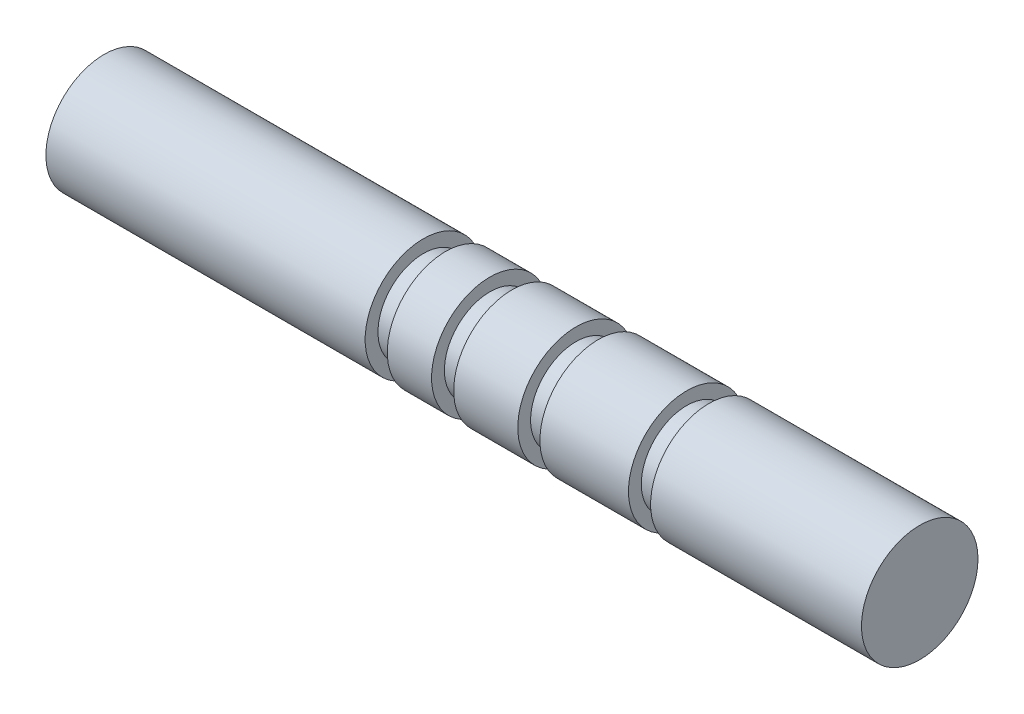
ISO-10303-21;
HEADER;
FILE_DESCRIPTION(('STEP AP214'),'2;1');
FILE_NAME('part.step','',(''),(''),'','','');
FILE_SCHEMA(('AUTOMOTIVE_DESIGN { 1 0 10303 214 1 1 1 1 }'));
ENDSEC;
DATA;
#1=APPLICATION_CONTEXT('core data for automotive mechanical design processes');
#2=APPLICATION_PROTOCOL_DEFINITION('international standard','automotive_design',2000,#1);
#3=PRODUCT_CONTEXT('',#1,'mechanical');
#4=PRODUCT('Part','Part','',(#3));
#5=PRODUCT_RELATED_PRODUCT_CATEGORY('part','',(#4));
#6=PRODUCT_DEFINITION_FORMATION('','',#4);
#7=PRODUCT_DEFINITION_CONTEXT('part definition',#1,'design');
#8=PRODUCT_DEFINITION('design','',#6,#7);
#9=PRODUCT_DEFINITION_SHAPE('','',#8);
#10=(LENGTH_UNIT() NAMED_UNIT(*) SI_UNIT(.MILLI.,.METRE.));
#11=(NAMED_UNIT(*) PLANE_ANGLE_UNIT() SI_UNIT($,.RADIAN.));
#12=(NAMED_UNIT(*) SI_UNIT($,.STERADIAN.) SOLID_ANGLE_UNIT());
#13=UNCERTAINTY_MEASURE_WITH_UNIT(LENGTH_MEASURE(1.E-05),#10,'distance_accuracy_value','');
#14=(GEOMETRIC_REPRESENTATION_CONTEXT(3) GLOBAL_UNCERTAINTY_ASSIGNED_CONTEXT((#13)) GLOBAL_UNIT_ASSIGNED_CONTEXT((#10,
#11,#12)) REPRESENTATION_CONTEXT('',''));
#15=CARTESIAN_POINT('',(0.,0.,0.));
#16=DIRECTION('',(0.,0.,1.));
#17=DIRECTION('',(1.,0.,0.));
#18=AXIS2_PLACEMENT_3D('',#15,#16,#17);
#19=CARTESIAN_POINT('',(-44.45,0.,0.));
#20=DIRECTION('',(-1.,0.,0.));
#21=DIRECTION('',(0.,0.,1.));
#22=AXIS2_PLACEMENT_3D('',#19,#20,#21);
#23=PLANE('',#22);
#24=CARTESIAN_POINT('',(-44.45,0.,0.));
#25=DIRECTION('',(1.,0.,0.));
#26=DIRECTION('',(0.,0.,-1.));
#27=AXIS2_PLACEMENT_3D('',#24,#25,#26);
#28=CIRCLE('',#27,6.34999999999999);
#29=CARTESIAN_POINT('',(-44.45,0.,-6.34999999999999));
#30=VERTEX_POINT('',#29);
#31=EDGE_CURVE('E10',#30,#30,#28,.T.);
#32=ORIENTED_EDGE('',*,*,#31,.F.);
#33=EDGE_LOOP('',(#32));
#34=FACE_BOUND('',#33,.T.);
#35=ADVANCED_FACE('F40',(#34),#23,.T.);
#36=CARTESIAN_POINT('',(49.9913538873995,0.,0.));
#37=DIRECTION('',(1.,0.,0.));
#38=DIRECTION('',(0.,0.,-1.));
#39=AXIS2_PLACEMENT_3D('',#36,#37,#38);
#40=CYLINDRICAL_SURFACE('',#39,6.34999999999999);
#41=ORIENTED_EDGE('',*,*,#31,.T.);
#42=EDGE_LOOP('',(#41));
#43=FACE_BOUND('',#42,.T.);
#44=CARTESIAN_POINT('',(-9.652,0.,0.));
#45=DIRECTION('',(1.,0.,0.));
#46=DIRECTION('',(0.,0.,-1.));
#47=AXIS2_PLACEMENT_3D('',#44,#45,#46);
#48=CIRCLE('',#47,6.34999999999999);
#49=CARTESIAN_POINT('',(-9.652,0.,-6.34999999999999));
#50=VERTEX_POINT('',#49);
#51=EDGE_CURVE('E43',#50,#50,#48,.T.);
#52=ORIENTED_EDGE('',*,*,#51,.F.);
#53=EDGE_LOOP('',(#52));
#54=FACE_BOUND('',#53,.T.);
#55=ADVANCED_FACE('F113',(#43,#54),#40,.T.);
#56=CARTESIAN_POINT('',(-9.652,6.34999999999999,0.));
#57=DIRECTION('',(1.,0.,0.));
#58=DIRECTION('',(0.,0.,-1.));
#59=AXIS2_PLACEMENT_3D('',#56,#57,#58);
#60=PLANE('',#59);
#61=ORIENTED_EDGE('',*,*,#51,.T.);
#62=EDGE_LOOP('',(#61));
#63=FACE_BOUND('',#62,.T.);
#64=CARTESIAN_POINT('',(-9.652,0.,0.));
#65=DIRECTION('',(1.,0.,0.));
#66=DIRECTION('',(0.,0.,-1.));
#67=AXIS2_PLACEMENT_3D('',#64,#65,#66);
#68=CIRCLE('',#67,4.95299999999999);
#69=CARTESIAN_POINT('',(-9.652,0.,-4.95299999999999));
#70=VERTEX_POINT('',#69);
#71=EDGE_CURVE('E50',#70,#70,#68,.T.);
#72=ORIENTED_EDGE('',*,*,#71,.F.);
#73=EDGE_LOOP('',(#72));
#74=FACE_BOUND('',#73,.T.);
#75=ADVANCED_FACE('F118',(#63,#74),#60,.T.);
#76=CARTESIAN_POINT('',(49.9913538873995,0.,0.));
#77=DIRECTION('',(1.,0.,0.));
#78=DIRECTION('',(0.,0.,-1.));
#79=AXIS2_PLACEMENT_3D('',#76,#77,#78);
#80=CYLINDRICAL_SURFACE('',#79,4.95299999999999);
#81=ORIENTED_EDGE('',*,*,#71,.T.);
#82=EDGE_LOOP('',(#81));
#83=FACE_BOUND('',#82,.T.);
#84=CARTESIAN_POINT('',(-7.239,0.,0.));
#85=DIRECTION('',(1.,0.,0.));
#86=DIRECTION('',(0.,0.,-1.));
#87=AXIS2_PLACEMENT_3D('',#84,#85,#86);
#88=CIRCLE('',#87,4.95299999999999);
#89=CARTESIAN_POINT('',(-7.239,0.,-4.95299999999999));
#90=VERTEX_POINT('',#89);
#91=EDGE_CURVE('E51',#90,#90,#88,.T.);
#92=ORIENTED_EDGE('',*,*,#91,.F.);
#93=EDGE_LOOP('',(#92));
#94=FACE_BOUND('',#93,.T.);
#95=ADVANCED_FACE('F122',(#83,#94),#80,.T.);
#96=CARTESIAN_POINT('',(-7.239,4.95299999999999,0.));
#97=DIRECTION('',(-1.,0.,0.));
#98=DIRECTION('',(0.,0.,1.));
#99=AXIS2_PLACEMENT_3D('',#96,#97,#98);
#100=PLANE('',#99);
#101=ORIENTED_EDGE('',*,*,#91,.T.);
#102=EDGE_LOOP('',(#101));
#103=FACE_BOUND('',#102,.T.);
#104=CARTESIAN_POINT('',(-7.239,0.,0.));
#105=DIRECTION('',(1.,0.,0.));
#106=DIRECTION('',(0.,0.,-1.));
#107=AXIS2_PLACEMENT_3D('',#104,#105,#106);
#108=CIRCLE('',#107,6.34999999999999);
#109=CARTESIAN_POINT('',(-7.239,0.,-6.34999999999999));
#110=VERTEX_POINT('',#109);
#111=EDGE_CURVE('E57',#110,#110,#108,.T.);
#112=ORIENTED_EDGE('',*,*,#111,.F.);
#113=EDGE_LOOP('',(#112));
#114=FACE_BOUND('',#113,.T.);
#115=ADVANCED_FACE('F128',(#103,#114),#100,.T.);
#116=CARTESIAN_POINT('',(49.9913538873995,0.,0.));
#117=DIRECTION('',(1.,0.,0.));
#118=DIRECTION('',(0.,0.,-1.));
#119=AXIS2_PLACEMENT_3D('',#116,#117,#118);
#120=CYLINDRICAL_SURFACE('',#119,6.34999999999999);
#121=ORIENTED_EDGE('',*,*,#111,.T.);
#122=EDGE_LOOP('',(#121));
#123=FACE_BOUND('',#122,.T.);
#124=CARTESIAN_POINT('',(-2.413,0.,0.));
#125=DIRECTION('',(1.,0.,0.));
#126=DIRECTION('',(0.,0.,-1.));
#127=AXIS2_PLACEMENT_3D('',#124,#125,#126);
#128=CIRCLE('',#127,6.34999999999999);
#129=CARTESIAN_POINT('',(-2.413,0.,-6.34999999999999));
#130=VERTEX_POINT('',#129);
#131=EDGE_CURVE('E56',#130,#130,#128,.T.);
#132=ORIENTED_EDGE('',*,*,#131,.F.);
#133=EDGE_LOOP('',(#132));
#134=FACE_BOUND('',#133,.T.);
#135=ADVANCED_FACE('F131',(#123,#134),#120,.T.);
#136=CARTESIAN_POINT('',(-2.413,6.34999999999999,0.));
#137=DIRECTION('',(1.,0.,0.));
#138=DIRECTION('',(0.,0.,-1.));
#139=AXIS2_PLACEMENT_3D('',#136,#137,#138);
#140=PLANE('',#139);
#141=ORIENTED_EDGE('',*,*,#131,.T.);
#142=EDGE_LOOP('',(#141));
#143=FACE_BOUND('',#142,.T.);
#144=CARTESIAN_POINT('',(-2.413,0.,0.));
#145=DIRECTION('',(1.,0.,0.));
#146=DIRECTION('',(0.,0.,-1.));
#147=AXIS2_PLACEMENT_3D('',#144,#145,#146);
#148=CIRCLE('',#147,4.95299999999999);
#149=CARTESIAN_POINT('',(-2.413,0.,-4.95299999999999));
#150=VERTEX_POINT('',#149);
#151=EDGE_CURVE('E65',#150,#150,#148,.T.);
#152=ORIENTED_EDGE('',*,*,#151,.F.);
#153=EDGE_LOOP('',(#152));
#154=FACE_BOUND('',#153,.T.);
#155=ADVANCED_FACE('F138',(#143,#154),#140,.T.);
#156=CARTESIAN_POINT('',(49.9913538873995,0.,0.));
#157=DIRECTION('',(1.,0.,0.));
#158=DIRECTION('',(0.,0.,-1.));
#159=AXIS2_PLACEMENT_3D('',#156,#157,#158);
#160=CYLINDRICAL_SURFACE('',#159,4.95299999999999);
#161=ORIENTED_EDGE('',*,*,#151,.T.);
#162=EDGE_LOOP('',(#161));
#163=FACE_BOUND('',#162,.T.);
#164=CARTESIAN_POINT('',(0.,0.,0.));
#165=DIRECTION('',(1.,0.,0.));
#166=DIRECTION('',(0.,0.,-1.));
#167=AXIS2_PLACEMENT_3D('',#164,#165,#166);
#168=CIRCLE('',#167,4.95299999999999);
#169=CARTESIAN_POINT('',(0.,0.,-4.95299999999999));
#170=VERTEX_POINT('',#169);
#171=EDGE_CURVE('E63',#170,#170,#168,.T.);
#172=ORIENTED_EDGE('',*,*,#171,.F.);
#173=EDGE_LOOP('',(#172));
#174=FACE_BOUND('',#173,.T.);
#175=ADVANCED_FACE('F142',(#163,#174),#160,.T.);
#176=CARTESIAN_POINT('',(0.,4.95299999999999,0.));
#177=DIRECTION('',(-1.,0.,0.));
#178=DIRECTION('',(0.,0.,1.));
#179=AXIS2_PLACEMENT_3D('',#176,#177,#178);
#180=PLANE('',#179);
#181=ORIENTED_EDGE('',*,*,#171,.T.);
#182=EDGE_LOOP('',(#181));
#183=FACE_BOUND('',#182,.T.);
#184=CARTESIAN_POINT('',(0.,0.,0.));
#185=DIRECTION('',(1.,0.,0.));
#186=DIRECTION('',(0.,0.,-1.));
#187=AXIS2_PLACEMENT_3D('',#184,#185,#186);
#188=CIRCLE('',#187,6.34999999999999);
#189=CARTESIAN_POINT('',(0.,0.,-6.34999999999999));
#190=VERTEX_POINT('',#189);
#191=EDGE_CURVE('E68',#190,#190,#188,.T.);
#192=ORIENTED_EDGE('',*,*,#191,.F.);
#193=EDGE_LOOP('',(#192));
#194=FACE_BOUND('',#193,.T.);
#195=ADVANCED_FACE('F148',(#183,#194),#180,.T.);
#196=CARTESIAN_POINT('',(49.9913538873995,0.,0.));
#197=DIRECTION('',(1.,0.,0.));
#198=DIRECTION('',(0.,0.,-1.));
#199=AXIS2_PLACEMENT_3D('',#196,#197,#198);
#200=CYLINDRICAL_SURFACE('',#199,6.34999999999999);
#201=ORIENTED_EDGE('',*,*,#191,.T.);
#202=EDGE_LOOP('',(#201));
#203=FACE_BOUND('',#202,.T.);
#204=CARTESIAN_POINT('',(6.985,0.,0.));
#205=DIRECTION('',(1.,0.,0.));
#206=DIRECTION('',(0.,0.,-1.));
#207=AXIS2_PLACEMENT_3D('',#204,#205,#206);
#208=CIRCLE('',#207,6.34999999999999);
#209=CARTESIAN_POINT('',(6.985,0.,-6.34999999999999));
#210=VERTEX_POINT('',#209);
#211=EDGE_CURVE('E72',#210,#210,#208,.T.);
#212=ORIENTED_EDGE('',*,*,#211,.F.);
#213=EDGE_LOOP('',(#212));
#214=FACE_BOUND('',#213,.T.);
#215=ADVANCED_FACE('F147',(#203,#214),#200,.T.);
#216=CARTESIAN_POINT('',(6.985,6.34999999999999,0.));
#217=DIRECTION('',(1.,0.,0.));
#218=DIRECTION('',(0.,0.,-1.));
#219=AXIS2_PLACEMENT_3D('',#216,#217,#218);
#220=PLANE('',#219);
#221=ORIENTED_EDGE('',*,*,#211,.T.);
#222=EDGE_LOOP('',(#221));
#223=FACE_BOUND('',#222,.T.);
#224=CARTESIAN_POINT('',(6.985,0.,0.));
#225=DIRECTION('',(1.,0.,0.));
#226=DIRECTION('',(0.,0.,-1.));
#227=AXIS2_PLACEMENT_3D('',#224,#225,#226);
#228=CIRCLE('',#227,4.95299999999999);
#229=CARTESIAN_POINT('',(6.985,0.,-4.95299999999999));
#230=VERTEX_POINT('',#229);
#231=EDGE_CURVE('E74',#230,#230,#228,.T.);
#232=ORIENTED_EDGE('',*,*,#231,.F.);
#233=EDGE_LOOP('',(#232));
#234=FACE_BOUND('',#233,.T.);
#235=ADVANCED_FACE('F152',(#223,#234),#220,.T.);
#236=CARTESIAN_POINT('',(49.9913538873995,0.,0.));
#237=DIRECTION('',(1.,0.,0.));
#238=DIRECTION('',(0.,0.,-1.));
#239=AXIS2_PLACEMENT_3D('',#236,#237,#238);
#240=CYLINDRICAL_SURFACE('',#239,4.95299999999999);
#241=ORIENTED_EDGE('',*,*,#231,.T.);
#242=EDGE_LOOP('',(#241));
#243=FACE_BOUND('',#242,.T.);
#244=CARTESIAN_POINT('',(9.398,0.,0.));
#245=DIRECTION('',(1.,0.,0.));
#246=DIRECTION('',(0.,0.,-1.));
#247=AXIS2_PLACEMENT_3D('',#244,#245,#246);
#248=CIRCLE('',#247,4.95299999999999);
#249=CARTESIAN_POINT('',(9.398,0.,-4.95299999999999));
#250=VERTEX_POINT('',#249);
#251=EDGE_CURVE('E80',#250,#250,#248,.T.);
#252=ORIENTED_EDGE('',*,*,#251,.F.);
#253=EDGE_LOOP('',(#252));
#254=FACE_BOUND('',#253,.T.);
#255=ADVANCED_FACE('F158',(#243,#254),#240,.T.);
#256=CARTESIAN_POINT('',(9.398,4.95299999999999,0.));
#257=DIRECTION('',(-1.,0.,0.));
#258=DIRECTION('',(0.,0.,1.));
#259=AXIS2_PLACEMENT_3D('',#256,#257,#258);
#260=PLANE('',#259);
#261=ORIENTED_EDGE('',*,*,#251,.T.);
#262=EDGE_LOOP('',(#261));
#263=FACE_BOUND('',#262,.T.);
#264=CARTESIAN_POINT('',(9.398,0.,0.));
#265=DIRECTION('',(1.,0.,0.));
#266=DIRECTION('',(0.,0.,-1.));
#267=AXIS2_PLACEMENT_3D('',#264,#265,#266);
#268=CIRCLE('',#267,6.34999999999999);
#269=CARTESIAN_POINT('',(9.398,0.,-6.34999999999999));
#270=VERTEX_POINT('',#269);
#271=EDGE_CURVE('E78',#270,#270,#268,.T.);
#272=ORIENTED_EDGE('',*,*,#271,.F.);
#273=EDGE_LOOP('',(#272));
#274=FACE_BOUND('',#273,.T.);
#275=ADVANCED_FACE('F165',(#263,#274),#260,.T.);
#276=CARTESIAN_POINT('',(49.9913538873995,0.,0.));
#277=DIRECTION('',(1.,0.,0.));
#278=DIRECTION('',(0.,0.,-1.));
#279=AXIS2_PLACEMENT_3D('',#276,#277,#278);
#280=CYLINDRICAL_SURFACE('',#279,6.34999999999999);
#281=ORIENTED_EDGE('',*,*,#271,.T.);
#282=EDGE_LOOP('',(#281));
#283=FACE_BOUND('',#282,.T.);
#284=CARTESIAN_POINT('',(19.05,0.,0.));
#285=DIRECTION('',(1.,0.,0.));
#286=DIRECTION('',(0.,0.,-1.));
#287=AXIS2_PLACEMENT_3D('',#284,#285,#286);
#288=CIRCLE('',#287,6.34999999999999);
#289=CARTESIAN_POINT('',(19.05,0.,-6.34999999999999));
#290=VERTEX_POINT('',#289);
#291=EDGE_CURVE('E83',#290,#290,#288,.T.);
#292=ORIENTED_EDGE('',*,*,#291,.F.);
#293=EDGE_LOOP('',(#292));
#294=FACE_BOUND('',#293,.T.);
#295=ADVANCED_FACE('F167',(#283,#294),#280,.T.);
#296=CARTESIAN_POINT('',(19.05,6.34999999999999,0.));
#297=DIRECTION('',(1.,0.,0.));
#298=DIRECTION('',(0.,0.,-1.));
#299=AXIS2_PLACEMENT_3D('',#296,#297,#298);
#300=PLANE('',#299);
#301=ORIENTED_EDGE('',*,*,#291,.T.);
#302=EDGE_LOOP('',(#301));
#303=FACE_BOUND('',#302,.T.);
#304=CARTESIAN_POINT('',(19.05,0.,0.));
#305=DIRECTION('',(1.,0.,0.));
#306=DIRECTION('',(0.,0.,-1.));
#307=AXIS2_PLACEMENT_3D('',#304,#305,#306);
#308=CIRCLE('',#307,4.95299999999999);
#309=CARTESIAN_POINT('',(19.05,0.,-4.95299999999999));
#310=VERTEX_POINT('',#309);
#311=EDGE_CURVE('E88',#310,#310,#308,.T.);
#312=ORIENTED_EDGE('',*,*,#311,.F.);
#313=EDGE_LOOP('',(#312));
#314=FACE_BOUND('',#313,.T.);
#315=ADVANCED_FACE('F168',(#303,#314),#300,.T.);
#316=CARTESIAN_POINT('',(49.9913538873995,0.,0.));
#317=DIRECTION('',(1.,0.,0.));
#318=DIRECTION('',(0.,0.,-1.));
#319=AXIS2_PLACEMENT_3D('',#316,#317,#318);
#320=CYLINDRICAL_SURFACE('',#319,4.95299999999999);
#321=ORIENTED_EDGE('',*,*,#311,.T.);
#322=EDGE_LOOP('',(#321));
#323=FACE_BOUND('',#322,.T.);
#324=CARTESIAN_POINT('',(21.463,0.,0.));
#325=DIRECTION('',(1.,0.,0.));
#326=DIRECTION('',(0.,0.,-1.));
#327=AXIS2_PLACEMENT_3D('',#324,#325,#326);
#328=CIRCLE('',#327,4.95299999999999);
#329=CARTESIAN_POINT('',(21.463,0.,-4.95299999999999));
#330=VERTEX_POINT('',#329);
#331=EDGE_CURVE('E90',#330,#330,#328,.T.);
#332=ORIENTED_EDGE('',*,*,#331,.F.);
#333=EDGE_LOOP('',(#332));
#334=FACE_BOUND('',#333,.T.);
#335=ADVANCED_FACE('F112',(#323,#334),#320,.T.);
#336=CARTESIAN_POINT('',(21.463,4.95299999999999,0.));
#337=DIRECTION('',(-1.,0.,0.));
#338=DIRECTION('',(0.,0.,1.));
#339=AXIS2_PLACEMENT_3D('',#336,#337,#338);
#340=PLANE('',#339);
#341=ORIENTED_EDGE('',*,*,#331,.T.);
#342=EDGE_LOOP('',(#341));
#343=FACE_BOUND('',#342,.T.);
#344=CARTESIAN_POINT('',(21.463,0.,0.));
#345=DIRECTION('',(1.,0.,0.));
#346=DIRECTION('',(0.,0.,-1.));
#347=AXIS2_PLACEMENT_3D('',#344,#345,#346);
#348=CIRCLE('',#347,6.34999999999999);
#349=CARTESIAN_POINT('',(21.463,0.,-6.34999999999999));
#350=VERTEX_POINT('',#349);
#351=EDGE_CURVE('E95',#350,#350,#348,.T.);
#352=ORIENTED_EDGE('',*,*,#351,.F.);
#353=EDGE_LOOP('',(#352));
#354=FACE_BOUND('',#353,.T.);
#355=ADVANCED_FACE('F103',(#343,#354),#340,.T.);
#356=CARTESIAN_POINT('',(49.9913538873995,0.,0.));
#357=DIRECTION('',(1.,0.,0.));
#358=DIRECTION('',(0.,0.,-1.));
#359=AXIS2_PLACEMENT_3D('',#356,#357,#358);
#360=CYLINDRICAL_SURFACE('',#359,6.34999999999999);
#361=ORIENTED_EDGE('',*,*,#351,.T.);
#362=EDGE_LOOP('',(#361));
#363=FACE_BOUND('',#362,.T.);
#364=CARTESIAN_POINT('',(44.45,0.,0.));
#365=DIRECTION('',(1.,0.,0.));
#366=DIRECTION('',(0.,0.,-1.));
#367=AXIS2_PLACEMENT_3D('',#364,#365,#366);
#368=CIRCLE('',#367,6.34999999999999);
#369=CARTESIAN_POINT('',(44.45,0.,-6.34999999999999));
#370=VERTEX_POINT('',#369);
#371=EDGE_CURVE('E92',#370,#370,#368,.T.);
#372=ORIENTED_EDGE('',*,*,#371,.F.);
#373=EDGE_LOOP('',(#372));
#374=FACE_BOUND('',#373,.T.);
#375=ADVANCED_FACE('F101',(#363,#374),#360,.T.);
#376=CARTESIAN_POINT('',(44.45,6.34999999999999,0.));
#377=DIRECTION('',(1.,0.,0.));
#378=DIRECTION('',(0.,0.,-1.));
#379=AXIS2_PLACEMENT_3D('',#376,#377,#378);
#380=PLANE('',#379);
#381=ORIENTED_EDGE('',*,*,#371,.T.);
#382=EDGE_LOOP('',(#381));
#383=FACE_BOUND('',#382,.T.);
#384=ADVANCED_FACE('F97',(#383),#380,.T.);
#385=CLOSED_SHELL('',(#35,#55,#75,#95,#115,#135,#155,#175,#195,#215,#235,#255,#275,#295,#315,
#335,#355,#375,#384));
#386=MANIFOLD_SOLID_BREP('B2',#385);
#387=ADVANCED_BREP_SHAPE_REPRESENTATION('',(#18,#386),#14);
#388=SHAPE_DEFINITION_REPRESENTATION(#9,#387);
ENDSEC;
END-ISO-10303-21;
